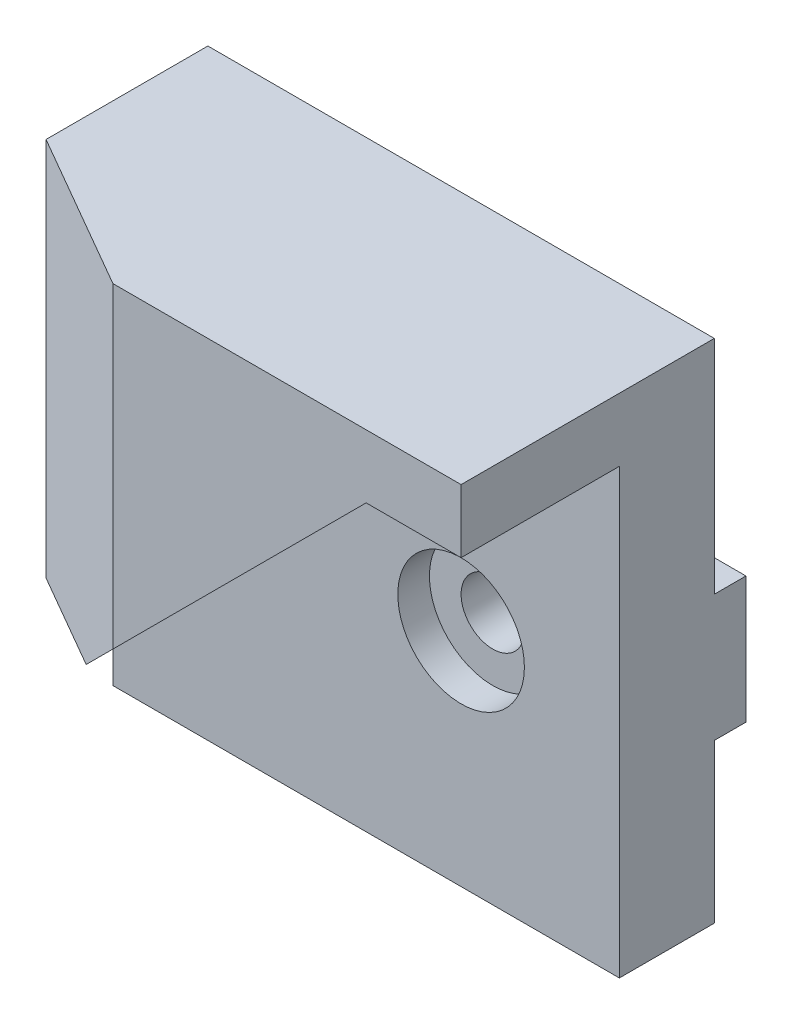
ISO-10303-21;
HEADER;
FILE_DESCRIPTION(('STEP AP214'),'2;1');
FILE_NAME('part.step','',(''),(''),'','','');
FILE_SCHEMA(('AUTOMOTIVE_DESIGN { 1 0 10303 214 1 1 1 1 }'));
ENDSEC;
DATA;
#1=APPLICATION_CONTEXT('core data for automotive mechanical design processes');
#2=APPLICATION_PROTOCOL_DEFINITION('international standard','automotive_design',2000,#1);
#3=PRODUCT_CONTEXT('',#1,'mechanical');
#4=PRODUCT('Part','Part','',(#3));
#5=PRODUCT_RELATED_PRODUCT_CATEGORY('part','',(#4));
#6=PRODUCT_DEFINITION_FORMATION('','',#4);
#7=PRODUCT_DEFINITION_CONTEXT('part definition',#1,'design');
#8=PRODUCT_DEFINITION('design','',#6,#7);
#9=PRODUCT_DEFINITION_SHAPE('','',#8);
#10=(LENGTH_UNIT() NAMED_UNIT(*) SI_UNIT(.MILLI.,.METRE.));
#11=(NAMED_UNIT(*) PLANE_ANGLE_UNIT() SI_UNIT($,.RADIAN.));
#12=(NAMED_UNIT(*) SI_UNIT($,.STERADIAN.) SOLID_ANGLE_UNIT());
#13=UNCERTAINTY_MEASURE_WITH_UNIT(LENGTH_MEASURE(1.E-05),#10,'distance_accuracy_value','');
#14=(GEOMETRIC_REPRESENTATION_CONTEXT(3) GLOBAL_UNCERTAINTY_ASSIGNED_CONTEXT((#13)) GLOBAL_UNIT_ASSIGNED_CONTEXT((#10,
#11,#12)) REPRESENTATION_CONTEXT('',''));
#15=CARTESIAN_POINT('',(0.,0.,0.));
#16=DIRECTION('',(0.,0.,1.));
#17=DIRECTION('',(1.,0.,0.));
#18=AXIS2_PLACEMENT_3D('',#15,#16,#17);
#19=CARTESIAN_POINT('',(0.,0.,0.));
#20=DIRECTION('',(0.,0.,-1.));
#21=DIRECTION('',(-1.,0.,0.));
#22=AXIS2_PLACEMENT_3D('',#19,#20,#21);
#23=PLANE('',#22);
#24=DIRECTION('',(0.,-1.,0.));
#25=VECTOR('',#24,1.);
#26=CARTESIAN_POINT('',(0.,-80.,0.));
#27=LINE('',#26,#25);
#28=CARTESIAN_POINT('',(0.,-55.,0.));
#29=VERTEX_POINT('',#28);
#30=CARTESIAN_POINT('',(0.,-80.,0.));
#31=VERTEX_POINT('',#30);
#32=EDGE_CURVE('E209',#29,#31,#27,.T.);
#33=ORIENTED_EDGE('',*,*,#32,.F.);
#34=DIRECTION('',(1.,0.,0.));
#35=VECTOR('',#34,1.);
#36=CARTESIAN_POINT('',(0.,-55.,0.));
#37=LINE('',#36,#35);
#38=CARTESIAN_POINT('',(80.,-55.,0.));
#39=VERTEX_POINT('',#38);
#40=EDGE_CURVE('E196',#29,#39,#37,.T.);
#41=ORIENTED_EDGE('',*,*,#40,.T.);
#42=DIRECTION('',(0.,1.,0.));
#43=VECTOR('',#42,1.);
#44=CARTESIAN_POINT('',(80.,0.,0.));
#45=LINE('',#44,#43);
#46=CARTESIAN_POINT('',(80.,-80.,0.));
#47=VERTEX_POINT('',#46);
#48=EDGE_CURVE('E230',#47,#39,#45,.T.);
#49=ORIENTED_EDGE('',*,*,#48,.F.);
#50=DIRECTION('',(1.,0.,0.));
#51=VECTOR('',#50,1.);
#52=CARTESIAN_POINT('',(80.,-80.,0.));
#53=LINE('',#52,#51);
#54=EDGE_CURVE('E228',#31,#47,#53,.T.);
#55=ORIENTED_EDGE('',*,*,#54,.F.);
#56=EDGE_LOOP('',(#33,#41,#49,#55));
#57=FACE_BOUND('',#56,.T.);
#58=ADVANCED_FACE('F44',(#57),#23,.T.);
#59=CARTESIAN_POINT('',(0.,-80.,15.));
#60=DIRECTION('',(1.,0.,0.));
#61=DIRECTION('',(0.,0.,-1.));
#62=AXIS2_PLACEMENT_3D('',#59,#60,#61);
#63=PLANE('',#62);
#64=CARTESIAN_POINT('',(0.,0.,0.));
#65=VERTEX_POINT('',#64);
#66=CARTESIAN_POINT('',(0.,-35.,0.));
#67=VERTEX_POINT('',#66);
#68=EDGE_CURVE('E222',#65,#67,#27,.T.);
#69=ORIENTED_EDGE('',*,*,#68,.T.);
#70=DIRECTION('',(0.,0.,1.));
#71=VECTOR('',#70,1.);
#72=CARTESIAN_POINT('',(0.,-35.,-5.));
#73=LINE('',#72,#71);
#74=CARTESIAN_POINT('',(0.,-35.,-5.));
#75=VERTEX_POINT('',#74);
#76=EDGE_CURVE('E198',#75,#67,#73,.T.);
#77=ORIENTED_EDGE('',*,*,#76,.F.);
#78=DIRECTION('',(0.,1.,0.));
#79=VECTOR('',#78,1.);
#80=CARTESIAN_POINT('',(0.,-55.,-5.));
#81=LINE('',#80,#79);
#82=CARTESIAN_POINT('',(0.,-55.,-5.));
#83=VERTEX_POINT('',#82);
#84=EDGE_CURVE('E191',#83,#75,#81,.T.);
#85=ORIENTED_EDGE('',*,*,#84,.F.);
#86=DIRECTION('',(0.,0.,-1.));
#87=VECTOR('',#86,1.);
#88=CARTESIAN_POINT('',(0.,-55.,0.));
#89=LINE('',#88,#87);
#90=EDGE_CURVE('E192',#29,#83,#89,.T.);
#91=ORIENTED_EDGE('',*,*,#90,.F.);
#92=ORIENTED_EDGE('',*,*,#32,.T.);
#93=DIRECTION('',(0.,0.,-1.));
#94=VECTOR('',#93,1.);
#95=CARTESIAN_POINT('',(0.,-80.,15.));
#96=LINE('',#95,#94);
#97=CARTESIAN_POINT('',(0.,-80.,15.));
#98=VERTEX_POINT('',#97);
#99=EDGE_CURVE('E11',#98,#31,#96,.T.);
#100=ORIENTED_EDGE('',*,*,#99,.F.);
#101=DIRECTION('',(0.,-1.,0.));
#102=VECTOR('',#101,1.);
#103=CARTESIAN_POINT('',(0.,-80.,15.));
#104=LINE('',#103,#102);
#105=CARTESIAN_POINT('',(0.,-60.,15.));
#106=VERTEX_POINT('',#105);
#107=EDGE_CURVE('E213',#106,#98,#104,.T.);
#108=ORIENTED_EDGE('',*,*,#107,.F.);
#109=DIRECTION('',(0.,0.,1.));
#110=VECTOR('',#109,1.);
#111=CARTESIAN_POINT('',(0.,-60.,15.));
#112=LINE('',#111,#110);
#113=CARTESIAN_POINT('',(0.,-60.,25.5662432702593));
#114=VERTEX_POINT('',#113);
#115=EDGE_CURVE('E162',#106,#114,#112,.T.);
#116=ORIENTED_EDGE('',*,*,#115,.T.);
#117=DIRECTION('',(0.,1.,0.));
#118=VECTOR('',#117,1.);
#119=CARTESIAN_POINT('',(0.,-60.,25.5662432702593));
#120=LINE('',#119,#118);
#121=CARTESIAN_POINT('',(0.,0.,25.5662432702593));
#122=VERTEX_POINT('',#121);
#123=EDGE_CURVE('E175',#114,#122,#120,.T.);
#124=ORIENTED_EDGE('',*,*,#123,.T.);
#125=DIRECTION('',(0.,0.,-1.));
#126=VECTOR('',#125,1.);
#127=CARTESIAN_POINT('',(0.,0.,15.));
#128=LINE('',#127,#126);
#129=EDGE_CURVE('E225',#122,#65,#128,.T.);
#130=ORIENTED_EDGE('',*,*,#129,.T.);
#131=EDGE_LOOP('',(#69,#77,#85,#91,#92,#100,#108,#116,#124,#130));
#132=FACE_BOUND('',#131,.T.);
#133=ADVANCED_FACE('F50',(#132),#63,.F.);
#134=CARTESIAN_POINT('',(80.,-80.,15.));
#135=DIRECTION('',(0.,1.,0.));
#136=DIRECTION('',(0.,0.,1.));
#137=AXIS2_PLACEMENT_3D('',#134,#135,#136);
#138=PLANE('',#137);
#139=ORIENTED_EDGE('',*,*,#54,.T.);
#140=DIRECTION('',(0.,0.,-1.));
#141=VECTOR('',#140,1.);
#142=CARTESIAN_POINT('',(80.,-80.,15.));
#143=LINE('',#142,#141);
#144=CARTESIAN_POINT('',(80.,-80.,15.));
#145=VERTEX_POINT('',#144);
#146=EDGE_CURVE('E53',#145,#47,#143,.T.);
#147=ORIENTED_EDGE('',*,*,#146,.F.);
#148=DIRECTION('',(1.,0.,0.));
#149=VECTOR('',#148,1.);
#150=CARTESIAN_POINT('',(80.,-80.,15.));
#151=LINE('',#150,#149);
#152=EDGE_CURVE('E220',#98,#145,#151,.T.);
#153=ORIENTED_EDGE('',*,*,#152,.F.);
#154=ORIENTED_EDGE('',*,*,#99,.T.);
#155=EDGE_LOOP('',(#139,#147,#153,#154));
#156=FACE_BOUND('',#155,.T.);
#157=ADVANCED_FACE('F276',(#156),#138,.F.);
#158=CARTESIAN_POINT('',(80.,0.,15.));
#159=DIRECTION('',(-1.,0.,0.));
#160=DIRECTION('',(0.,0.,1.));
#161=AXIS2_PLACEMENT_3D('',#158,#159,#160);
#162=PLANE('',#161);
#163=ORIENTED_EDGE('',*,*,#48,.T.);
#164=DIRECTION('',(0.,0.,-1.));
#165=VECTOR('',#164,1.);
#166=CARTESIAN_POINT('',(80.,-55.,0.));
#167=LINE('',#166,#165);
#168=CARTESIAN_POINT('',(80.,-55.,-5.));
#169=VERTEX_POINT('',#168);
#170=EDGE_CURVE('E69',#39,#169,#167,.T.);
#171=ORIENTED_EDGE('',*,*,#170,.T.);
#172=DIRECTION('',(0.,1.,0.));
#173=VECTOR('',#172,1.);
#174=CARTESIAN_POINT('',(80.,-55.,-5.));
#175=LINE('',#174,#173);
#176=CARTESIAN_POINT('',(80.,-35.,-5.));
#177=VERTEX_POINT('',#176);
#178=EDGE_CURVE('E205',#169,#177,#175,.T.);
#179=ORIENTED_EDGE('',*,*,#178,.T.);
#180=DIRECTION('',(0.,0.,1.));
#181=VECTOR('',#180,1.);
#182=CARTESIAN_POINT('',(80.,-35.,-5.));
#183=LINE('',#182,#181);
#184=CARTESIAN_POINT('',(80.,-35.,0.));
#185=VERTEX_POINT('',#184);
#186=EDGE_CURVE('E193',#177,#185,#183,.T.);
#187=ORIENTED_EDGE('',*,*,#186,.T.);
#188=CARTESIAN_POINT('',(80.,0.,0.));
#189=VERTEX_POINT('',#188);
#190=EDGE_CURVE('E226',#185,#189,#45,.T.);
#191=ORIENTED_EDGE('',*,*,#190,.T.);
#192=DIRECTION('',(0.,0.,-1.));
#193=VECTOR('',#192,1.);
#194=CARTESIAN_POINT('',(80.,0.,15.));
#195=LINE('',#194,#193);
#196=CARTESIAN_POINT('',(80.,0.,40.));
#197=VERTEX_POINT('',#196);
#198=EDGE_CURVE('E232',#197,#189,#195,.T.);
#199=ORIENTED_EDGE('',*,*,#198,.F.);
#200=DIRECTION('',(0.,1.,0.));
#201=VECTOR('',#200,1.);
#202=CARTESIAN_POINT('',(80.,-10.,40.));
#203=LINE('',#202,#201);
#204=CARTESIAN_POINT('',(80.,-10.,40.));
#205=VERTEX_POINT('',#204);
#206=EDGE_CURVE('E187',#205,#197,#203,.T.);
#207=ORIENTED_EDGE('',*,*,#206,.F.);
#208=DIRECTION('',(0.,0.,-1.));
#209=VECTOR('',#208,1.);
#210=CARTESIAN_POINT('',(80.,-10.,15.));
#211=LINE('',#210,#209);
#212=CARTESIAN_POINT('',(80.,-10.,15.));
#213=VERTEX_POINT('',#212);
#214=EDGE_CURVE('E179',#205,#213,#211,.T.);
#215=ORIENTED_EDGE('',*,*,#214,.T.);
#216=DIRECTION('',(0.,1.,0.));
#217=VECTOR('',#216,1.);
#218=CARTESIAN_POINT('',(80.,0.,15.));
#219=LINE('',#218,#217);
#220=EDGE_CURVE('E216',#145,#213,#219,.T.);
#221=ORIENTED_EDGE('',*,*,#220,.F.);
#222=ORIENTED_EDGE('',*,*,#146,.T.);
#223=EDGE_LOOP('',(#163,#171,#179,#187,#191,#199,#207,#215,#221,#222));
#224=FACE_BOUND('',#223,.T.);
#225=ADVANCED_FACE('F243',(#224),#162,.F.);
#226=CARTESIAN_POINT('',(0.,0.,15.));
#227=DIRECTION('',(0.,-1.,0.));
#228=DIRECTION('',(0.,0.,-1.));
#229=AXIS2_PLACEMENT_3D('',#226,#227,#228);
#230=PLANE('',#229);
#231=ORIENTED_EDGE('',*,*,#129,.F.);
#232=DIRECTION('',(0.866025403784438,0.,0.500000000000001));
#233=VECTOR('',#232,1.);
#234=CARTESIAN_POINT('',(25.,0.,40.));
#235=LINE('',#234,#233);
#236=CARTESIAN_POINT('',(25.,0.,40.));
#237=VERTEX_POINT('',#236);
#238=EDGE_CURVE('E161',#122,#237,#235,.T.);
#239=ORIENTED_EDGE('',*,*,#238,.T.);
#240=DIRECTION('',(1.,0.,0.));
#241=VECTOR('',#240,1.);
#242=CARTESIAN_POINT('',(25.,0.,40.));
#243=LINE('',#242,#241);
#244=EDGE_CURVE('E176',#237,#197,#243,.T.);
#245=ORIENTED_EDGE('',*,*,#244,.T.);
#246=ORIENTED_EDGE('',*,*,#198,.T.);
#247=DIRECTION('',(-1.,0.,0.));
#248=VECTOR('',#247,1.);
#249=CARTESIAN_POINT('',(0.,0.,0.));
#250=LINE('',#249,#248);
#251=EDGE_CURVE('E218',#189,#65,#250,.T.);
#252=ORIENTED_EDGE('',*,*,#251,.T.);
#253=EDGE_LOOP('',(#231,#239,#245,#246,#252));
#254=FACE_BOUND('',#253,.T.);
#255=ADVANCED_FACE('F268',(#254),#230,.F.);
#256=CARTESIAN_POINT('',(0.,0.,15.));
#257=DIRECTION('',(0.,0.,-1.));
#258=DIRECTION('',(-1.,0.,0.));
#259=AXIS2_PLACEMENT_3D('',#256,#257,#258);
#260=PLANE('',#259);
#261=CARTESIAN_POINT('',(55.,-45.,15.));
#262=DIRECTION('',(0.,0.,1.));
#263=DIRECTION('',(1.,0.,0.));
#264=AXIS2_PLACEMENT_3D('',#261,#262,#263);
#265=CIRCLE('',#264,10.);
#266=CARTESIAN_POINT('',(65.,-45.,15.));
#267=VERTEX_POINT('',#266);
#268=EDGE_CURVE('E284',#267,#267,#265,.T.);
#269=ORIENTED_EDGE('',*,*,#268,.F.);
#270=EDGE_LOOP('',(#269));
#271=FACE_BOUND('',#270,.T.);
#272=DIRECTION('',(0.70710678118654,0.707106781186555,0.));
#273=VECTOR('',#272,1.);
#274=CARTESIAN_POINT('',(31.3743240959377,-43.6256759040625,15.));
#275=LINE('',#274,#273);
#276=CARTESIAN_POINT('',(15.0000000000003,-60.,15.));
#277=VERTEX_POINT('',#276);
#278=CARTESIAN_POINT('',(65.,-10.,15.));
#279=VERTEX_POINT('',#278);
#280=EDGE_CURVE('E138',#277,#279,#275,.T.);
#281=ORIENTED_EDGE('',*,*,#280,.F.);
#282=DIRECTION('',(-1.,0.,0.));
#283=VECTOR('',#282,1.);
#284=CARTESIAN_POINT('',(0.,-60.,15.));
#285=LINE('',#284,#283);
#286=EDGE_CURVE('E62',#277,#106,#285,.T.);
#287=ORIENTED_EDGE('',*,*,#286,.T.);
#288=ORIENTED_EDGE('',*,*,#107,.T.);
#289=ORIENTED_EDGE('',*,*,#152,.T.);
#290=ORIENTED_EDGE('',*,*,#220,.T.);
#291=DIRECTION('',(-1.,0.,0.));
#292=VECTOR('',#291,1.);
#293=CARTESIAN_POINT('',(25.,-10.,15.));
#294=LINE('',#293,#292);
#295=EDGE_CURVE('E141',#213,#279,#294,.T.);
#296=ORIENTED_EDGE('',*,*,#295,.T.);
#297=EDGE_LOOP('',(#281,#287,#288,#289,#290,#296));
#298=FACE_BOUND('',#297,.T.);
#299=ADVANCED_FACE('F142',(#271,#298),#260,.F.);
#300=DIRECTION('',(1.,0.,0.));
#301=VECTOR('',#300,1.);
#302=CARTESIAN_POINT('',(0.,-35.,0.));
#303=LINE('',#302,#301);
#304=EDGE_CURVE('E210',#67,#185,#303,.T.);
#305=ORIENTED_EDGE('',*,*,#304,.F.);
#306=ORIENTED_EDGE('',*,*,#68,.F.);
#307=ORIENTED_EDGE('',*,*,#251,.F.);
#308=ORIENTED_EDGE('',*,*,#190,.F.);
#309=EDGE_LOOP('',(#305,#306,#307,#308));
#310=FACE_BOUND('',#309,.T.);
#311=ADVANCED_FACE('F261',(#310),#23,.T.);
#312=CARTESIAN_POINT('',(0.,-35.,-5.));
#313=DIRECTION('',(0.,1.,0.));
#314=DIRECTION('',(0.,0.,1.));
#315=AXIS2_PLACEMENT_3D('',#312,#313,#314);
#316=PLANE('',#315);
#317=ORIENTED_EDGE('',*,*,#186,.F.);
#318=DIRECTION('',(1.,0.,0.));
#319=VECTOR('',#318,1.);
#320=CARTESIAN_POINT('',(0.,-35.,-5.));
#321=LINE('',#320,#319);
#322=EDGE_CURVE('E208',#75,#177,#321,.T.);
#323=ORIENTED_EDGE('',*,*,#322,.F.);
#324=ORIENTED_EDGE('',*,*,#76,.T.);
#325=ORIENTED_EDGE('',*,*,#304,.T.);
#326=EDGE_LOOP('',(#317,#323,#324,#325));
#327=FACE_BOUND('',#326,.T.);
#328=ADVANCED_FACE('F262',(#327),#316,.T.);
#329=CARTESIAN_POINT('',(0.,-55.,-5.));
#330=DIRECTION('',(0.,0.,-1.));
#331=DIRECTION('',(-1.,0.,0.));
#332=AXIS2_PLACEMENT_3D('',#329,#330,#331);
#333=PLANE('',#332);
#334=CARTESIAN_POINT('',(55.,-45.,-5.));
#335=DIRECTION('',(0.,0.,-1.));
#336=DIRECTION('',(-1.,0.,0.));
#337=AXIS2_PLACEMENT_3D('',#334,#335,#336);
#338=CIRCLE('',#337,5.);
#339=CARTESIAN_POINT('',(50.,-45.,-5.));
#340=VERTEX_POINT('',#339);
#341=EDGE_CURVE('E47',#340,#340,#338,.T.);
#342=ORIENTED_EDGE('',*,*,#341,.F.);
#343=EDGE_LOOP('',(#342));
#344=FACE_BOUND('',#343,.T.);
#345=ORIENTED_EDGE('',*,*,#178,.F.);
#346=DIRECTION('',(1.,0.,0.));
#347=VECTOR('',#346,1.);
#348=CARTESIAN_POINT('',(0.,-55.,-5.));
#349=LINE('',#348,#347);
#350=EDGE_CURVE('E215',#83,#169,#349,.T.);
#351=ORIENTED_EDGE('',*,*,#350,.F.);
#352=ORIENTED_EDGE('',*,*,#84,.T.);
#353=ORIENTED_EDGE('',*,*,#322,.T.);
#354=EDGE_LOOP('',(#345,#351,#352,#353));
#355=FACE_BOUND('',#354,.T.);
#356=ADVANCED_FACE('F260',(#344,#355),#333,.T.);
#357=CARTESIAN_POINT('',(0.,-55.,0.));
#358=DIRECTION('',(0.,-1.,0.));
#359=DIRECTION('',(0.,0.,-1.));
#360=AXIS2_PLACEMENT_3D('',#357,#358,#359);
#361=PLANE('',#360);
#362=ORIENTED_EDGE('',*,*,#170,.F.);
#363=ORIENTED_EDGE('',*,*,#40,.F.);
#364=ORIENTED_EDGE('',*,*,#90,.T.);
#365=ORIENTED_EDGE('',*,*,#350,.T.);
#366=EDGE_LOOP('',(#362,#363,#364,#365));
#367=FACE_BOUND('',#366,.T.);
#368=ADVANCED_FACE('F249',(#367),#361,.T.);
#369=CARTESIAN_POINT('',(25.,-10.,40.));
#370=DIRECTION('',(0.,0.,1.));
#371=DIRECTION('',(1.,0.,0.));
#372=AXIS2_PLACEMENT_3D('',#369,#370,#371);
#373=PLANE('',#372);
#374=ORIENTED_EDGE('',*,*,#244,.F.);
#375=DIRECTION('',(0.,1.,0.));
#376=VECTOR('',#375,1.);
#377=CARTESIAN_POINT('',(25.,-10.,40.));
#378=LINE('',#377,#376);
#379=CARTESIAN_POINT('',(25.,-50.0000000000003,40.));
#380=VERTEX_POINT('',#379);
#381=EDGE_CURVE('E182',#380,#237,#378,.T.);
#382=ORIENTED_EDGE('',*,*,#381,.F.);
#383=DIRECTION('',(0.707106781186546,0.707106781186549,0.));
#384=VECTOR('',#383,1.);
#385=CARTESIAN_POINT('',(65.,-10.,40.));
#386=LINE('',#385,#384);
#387=CARTESIAN_POINT('',(65.,-10.,40.));
#388=VERTEX_POINT('',#387);
#389=EDGE_CURVE('E150',#380,#388,#386,.T.);
#390=ORIENTED_EDGE('',*,*,#389,.T.);
#391=DIRECTION('',(1.,0.,0.));
#392=VECTOR('',#391,1.);
#393=CARTESIAN_POINT('',(25.,-10.,40.));
#394=LINE('',#393,#392);
#395=EDGE_CURVE('E178',#388,#205,#394,.T.);
#396=ORIENTED_EDGE('',*,*,#395,.T.);
#397=ORIENTED_EDGE('',*,*,#206,.T.);
#398=EDGE_LOOP('',(#374,#382,#390,#396,#397));
#399=FACE_BOUND('',#398,.T.);
#400=ADVANCED_FACE('F271',(#399),#373,.T.);
#401=CARTESIAN_POINT('',(0.,-10.,0.));
#402=DIRECTION('',(0.,-1.,0.));
#403=DIRECTION('',(0.,0.,-1.));
#404=AXIS2_PLACEMENT_3D('',#401,#402,#403);
#405=PLANE('',#404);
#406=DIRECTION('',(0.,0.,1.));
#407=VECTOR('',#406,1.);
#408=CARTESIAN_POINT('',(65.,-10.,15.));
#409=LINE('',#408,#407);
#410=EDGE_CURVE('E147',#279,#388,#409,.T.);
#411=ORIENTED_EDGE('',*,*,#410,.F.);
#412=ORIENTED_EDGE('',*,*,#295,.F.);
#413=ORIENTED_EDGE('',*,*,#214,.F.);
#414=ORIENTED_EDGE('',*,*,#395,.F.);
#415=EDGE_LOOP('',(#411,#412,#413,#414));
#416=FACE_BOUND('',#415,.T.);
#417=ADVANCED_FACE('F279',(#416),#405,.T.);
#418=CARTESIAN_POINT('',(25.,-60.,40.));
#419=DIRECTION('',(-0.500000000000001,0.,0.866025403784438));
#420=DIRECTION('',(0.866025403784438,0.,0.500000000000001));
#421=AXIS2_PLACEMENT_3D('',#418,#419,#420);
#422=PLANE('',#421);
#423=DIRECTION('',(-0.654653670707975,-0.654653670707979,-0.377964473009227));
#424=VECTOR('',#423,1.);
#425=CARTESIAN_POINT('',(20.7142857142858,-54.2857142857145,37.5256417034731));
#426=LINE('',#425,#424);
#427=CARTESIAN_POINT('',(15.0000000000003,-60.,34.2264973081039));
#428=VERTEX_POINT('',#427);
#429=EDGE_CURVE('E153',#380,#428,#426,.T.);
#430=ORIENTED_EDGE('',*,*,#429,.F.);
#431=ORIENTED_EDGE('',*,*,#381,.T.);
#432=ORIENTED_EDGE('',*,*,#238,.F.);
#433=ORIENTED_EDGE('',*,*,#123,.F.);
#434=DIRECTION('',(0.866025403784438,0.,0.500000000000001));
#435=VECTOR('',#434,1.);
#436=CARTESIAN_POINT('',(25.,-60.,40.));
#437=LINE('',#436,#435);
#438=EDGE_CURVE('E164',#114,#428,#437,.T.);
#439=ORIENTED_EDGE('',*,*,#438,.T.);
#440=EDGE_LOOP('',(#430,#431,#432,#433,#439));
#441=FACE_BOUND('',#440,.T.);
#442=ADVANCED_FACE('F282',(#441),#422,.T.);
#443=CARTESIAN_POINT('',(0.,-60.,0.));
#444=DIRECTION('',(0.,1.,0.));
#445=DIRECTION('',(0.,0.,1.));
#446=AXIS2_PLACEMENT_3D('',#443,#444,#445);
#447=PLANE('',#446);
#448=ORIENTED_EDGE('',*,*,#286,.F.);
#449=DIRECTION('',(0.,0.,1.));
#450=VECTOR('',#449,1.);
#451=CARTESIAN_POINT('',(15.0000000000003,-60.,15.));
#452=LINE('',#451,#450);
#453=EDGE_CURVE('E148',#277,#428,#452,.T.);
#454=ORIENTED_EDGE('',*,*,#453,.T.);
#455=ORIENTED_EDGE('',*,*,#438,.F.);
#456=ORIENTED_EDGE('',*,*,#115,.F.);
#457=EDGE_LOOP('',(#448,#454,#455,#456));
#458=FACE_BOUND('',#457,.T.);
#459=ADVANCED_FACE('F159',(#458),#447,.F.);
#460=CARTESIAN_POINT('',(65.,-10.,15.));
#461=DIRECTION('',(0.707106781186549,-0.707106781186546,0.));
#462=DIRECTION('',(0.707106781186546,0.707106781186549,0.));
#463=AXIS2_PLACEMENT_3D('',#460,#461,#462);
#464=PLANE('',#463);
#465=ORIENTED_EDGE('',*,*,#389,.F.);
#466=ORIENTED_EDGE('',*,*,#429,.T.);
#467=ORIENTED_EDGE('',*,*,#453,.F.);
#468=ORIENTED_EDGE('',*,*,#280,.T.);
#469=ORIENTED_EDGE('',*,*,#410,.T.);
#470=EDGE_LOOP('',(#465,#466,#467,#468,#469));
#471=FACE_BOUND('',#470,.T.);
#472=ADVANCED_FACE('F155',(#471),#464,.T.);
#473=CARTESIAN_POINT('',(55.,-45.,10.));
#474=DIRECTION('',(0.,0.,1.));
#475=DIRECTION('',(1.,0.,0.));
#476=AXIS2_PLACEMENT_3D('',#473,#474,#475);
#477=CYLINDRICAL_SURFACE('',#476,10.);
#478=CARTESIAN_POINT('',(55.,-45.,10.));
#479=DIRECTION('',(0.,0.,1.));
#480=DIRECTION('',(1.,0.,0.));
#481=AXIS2_PLACEMENT_3D('',#478,#479,#480);
#482=CIRCLE('',#481,10.);
#483=CARTESIAN_POINT('',(65.,-45.,10.));
#484=VERTEX_POINT('',#483);
#485=EDGE_CURVE('E160',#484,#484,#482,.T.);
#486=ORIENTED_EDGE('',*,*,#485,.F.);
#487=EDGE_LOOP('',(#486));
#488=FACE_BOUND('',#487,.T.);
#489=ORIENTED_EDGE('',*,*,#268,.T.);
#490=EDGE_LOOP('',(#489));
#491=FACE_BOUND('',#490,.T.);
#492=ADVANCED_FACE('F330',(#488,#491),#477,.F.);
#493=CARTESIAN_POINT('',(0.,0.,10.));
#494=DIRECTION('',(0.,0.,1.));
#495=DIRECTION('',(1.,0.,0.));
#496=AXIS2_PLACEMENT_3D('',#493,#494,#495);
#497=PLANE('',#496);
#498=CARTESIAN_POINT('',(55.,-45.,10.));
#499=DIRECTION('',(0.,0.,1.));
#500=DIRECTION('',(1.,0.,0.));
#501=AXIS2_PLACEMENT_3D('',#498,#499,#500);
#502=CIRCLE('',#501,5.);
#503=CARTESIAN_POINT('',(60.,-45.,10.));
#504=VERTEX_POINT('',#503);
#505=EDGE_CURVE('E288',#504,#504,#502,.T.);
#506=ORIENTED_EDGE('',*,*,#505,.F.);
#507=EDGE_LOOP('',(#506));
#508=FACE_BOUND('',#507,.T.);
#509=ORIENTED_EDGE('',*,*,#485,.T.);
#510=EDGE_LOOP('',(#509));
#511=FACE_BOUND('',#510,.T.);
#512=ADVANCED_FACE('F329',(#508,#511),#497,.T.);
#513=CARTESIAN_POINT('',(55.,-45.,-10.));
#514=DIRECTION('',(0.,0.,1.));
#515=DIRECTION('',(1.,0.,0.));
#516=AXIS2_PLACEMENT_3D('',#513,#514,#515);
#517=CYLINDRICAL_SURFACE('',#516,5.);
#518=ORIENTED_EDGE('',*,*,#341,.T.);
#519=EDGE_LOOP('',(#518));
#520=FACE_BOUND('',#519,.T.);
#521=ORIENTED_EDGE('',*,*,#505,.T.);
#522=EDGE_LOOP('',(#521));
#523=FACE_BOUND('',#522,.T.);
#524=ADVANCED_FACE('F298',(#520,#523),#517,.F.);
#525=CLOSED_SHELL('',(#58,#133,#157,#225,#255,#299,#311,#328,#356,#368,#400,#417,#442,#459,#472,
#492,#512,#524));
#526=MANIFOLD_SOLID_BREP('B2',#525);
#527=ADVANCED_BREP_SHAPE_REPRESENTATION('',(#18,#526),#14);
#528=SHAPE_DEFINITION_REPRESENTATION(#9,#527);
ENDSEC;
END-ISO-10303-21;
